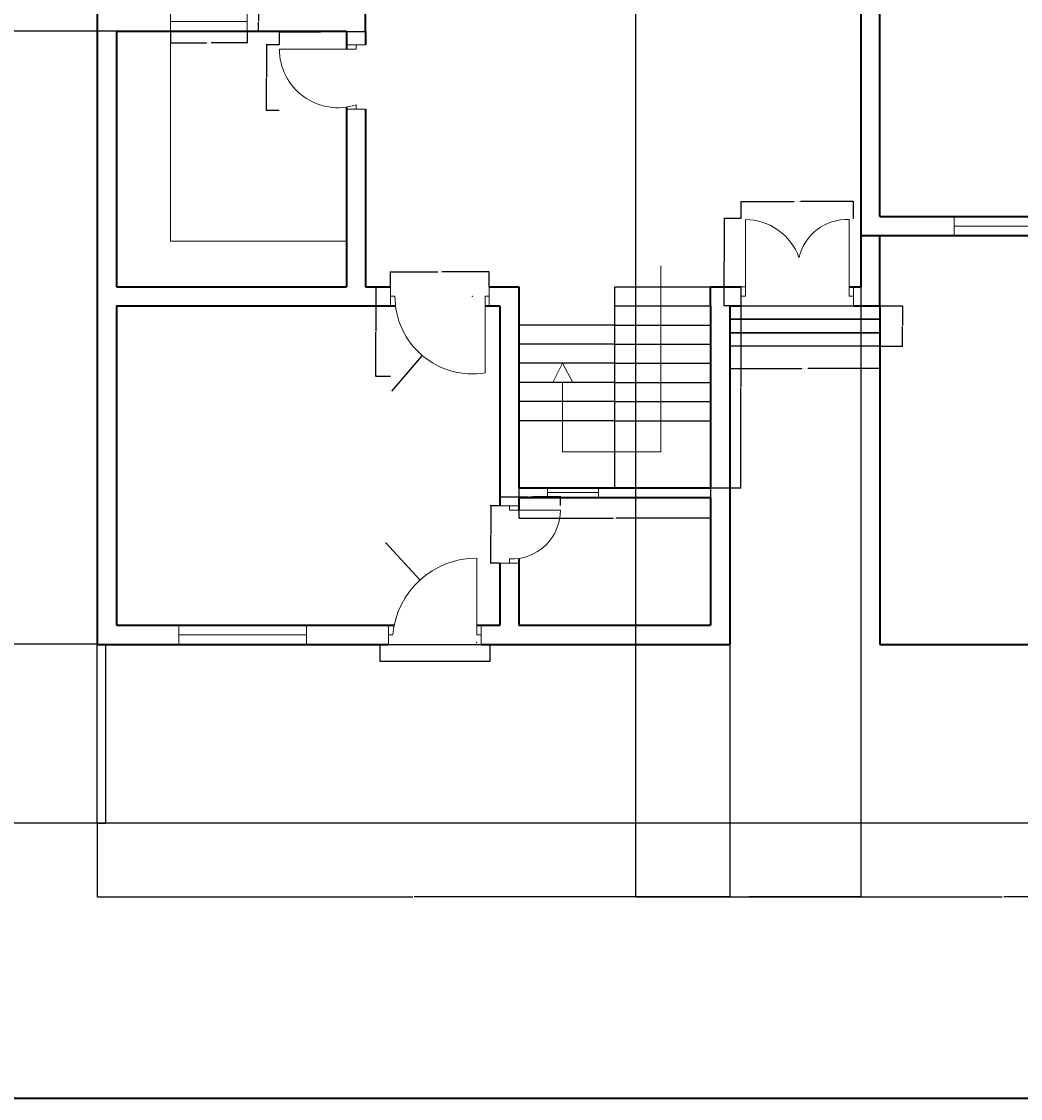
# Model space of a CAD drawing. Units: inches. Extents: x 2014 to 3678, y 870 to 2323.
# Tile 4 of 7: x 2813 to 3282, y 870 to 1376. Entities that reach past the tile are written whole.
import ezdxf

# ---------------------------------------------------------------- set-up
doc = ezdxf.new("R2010")
doc.units = ezdxf.units.IN
for name, color, linetype, lineweight in [('A-ANNO-DIMS', 2, 'Continuous', 18), ('A-ANNO-SYMB', 2, 'Continuous', 18), ('A-ANNO-TTLB', 7, 'Continuous', 35), ('A-DOOR', 3, 'Continuous', 18), ('A-FLOR-FIXT', 8, 'Continuous', 18), ('A-FLOR-STRS', 7, 'Continuous', 25), ('A-GLAZ', 4, 'Continuous', 18), ('A-SITE', 8, 'Continuous', 25), ('A-WALL', 7, 'Continuous', 35)]:
    doc.layers.add(name, color=color, linetype=linetype, lineweight=lineweight)
doc.styles.get("Standard").update_dxf_attribs({"font": 'arial.ttf'})
doc.dimstyles.get("Standard").update_dxf_attribs({"dimtxt": 0.18, "dimasz": 0.18, "dimexe": 0.18, "dimexo": 0.0625, "dimgap": 0.09, "dimtad": 0, "dimtih": 1, "dimtoh": 1, "dimdec": 4, "dimzin": 0, "dimdsep": 46, "dimtxsty": 'Standard', "dimcen": 0.09, "dimadec": 0, "dimazin": 0, "dimtfac": 1, "dimtdec": 4, "dimtofl": 0, "dimtmove": 0, "dimatfit": 3, "dimfxl": 1, "dimtolj": 1, "dimtzin": 0, "dimarcsym": 0})

# ---------------------------------------------------------------- blocks, each defined once
blk = doc.blocks.new('DOOR-DRAWING-36')
for p, q in [((0, 40.98), (0, 31.98)), ((46.34, 40.98), (46.34, 31.98)), ((0, 31.98), (0, 36.48)), ((0, 36.48), (2, 36.48)), ((46.34, 36.48), (44.34, 36.48)), ((44.34, 36.48), (44.34, 0.48)), ((46.34, 31.98), (46.34, 36.48))]:
    blk.add_line(p, q)
blk.add_arc((38.48, 36.48), 36.48, 180, 279.258)
blk = doc.blocks.new('DOOR-BATH-FRONT-24')
for p, q in [((0, 27), (9, 27)), ((9, 27), (4.5, 27)), ((4.5, 27), (4.5, 25)), ((4.5, 25), (28.5, 25)), ((4.5, 0), (4.5, 2)), ((0, 0), (9, 0)), ((9, 0), (4.5, 0))]:
    blk.add_line(p, q)
blk.add_arc((5.48, 25), 23.02, 267.569, 0)
blk = doc.blocks.new('DOOR-FRONT-36')
for p, q in [((41.48, 4.5), (41.48, 40.5)), ((0, 9), (0, 0)), ((43.48, 9), (43.48, 0)), ((0, 0), (0, 4.5)), ((0, 4.5), (2, 4.5)), ((43.48, 4.5), (41.48, 4.5)), ((43.48, 0), (43.48, 4.5))]:
    blk.add_line(p, q)
blk.add_arc((41.48, 0.85), 39.65, 90, 174.7231)
blk = doc.blocks.new('DOOR-KITCHEN-36')
for p, q in [((12, 28.21), (0, 28.21)), ((36, 28.21), (12, 28.21)), ((31.5, 30.21), (40.5, 30.21)), ((40.5, 30.21), (36, 30.21)), ((36, 30.21), (36, 28.21)), ((36, 0), (36, 2)), ((40.5, 0), (31.5, 0)), ((31.5, 0), (36, 0))]:
    blk.add_line(p, q)
blk.add_arc((27.54, 28.21), 27.54, 180, 287.8943)
blk = doc.blocks.new('WIN-60')
for p, q in [((0, 9), (0, 0)), ((60, 4.5), (60, 9)), ((60, 9), (60, 0)), ((0, 0), (0, 4.5)), ((0, 4.5), (60, 4.5))]:
    blk.add_line(p, q)
blk = doc.blocks.new('VENT-24')
for p, q in [((0, 24), (4.5, 24)), ((4.5, 24), (2.25, 24)), ((2.25, 24), (2.25, 0)), ((2.25, 0), (0, 0)), ((0, 0), (4.5, 0))]:
    blk.add_line(p, q)
blk = doc.blocks.new('WIN-36')
for p, q in [((0, 9), (0, 0)), ((36, 0), (36, 9)), ((0, 0), (0, 4.5)), ((0, 4.5), (36, 4.5)), ((36, 4.5), (36, 0))]:
    blk.add_line(p, q)
blk = doc.blocks.new('STAIR-HALF-TURN')
for p, q in [((45, 0), (45, 94.5)), ((45, 94.5), (90, 94.5)), ((45, 85.5), (90, 85.5)), ((45, 76.5), (0, 76.5)), ((45, 76.5), (90, 76.5)), ((45, 67.5), (0, 67.5)), ((45, 67.5), (90, 67.5)), ((45, 58.5), (0, 58.5)), ((45, 58.5), (90, 58.5)), ((45, 49.5), (0, 49.5)), ((45, 49.5), (90, 49.5)), ((45, 40.5), (0, 40.5)), ((45, 40.5), (90, 40.5)), ((45, 31.5), (0, 31.5)), ((45, 31.5), (90, 31.5)), ((90, 0), (0, 0))]:
    blk.add_line(p, q)
blk = doc.blocks.new('STAIR-DIRECTION')
for p, q in [((50.73, 87.32), (50.73, 0)), ((4.61, 41.51), (0, 32.51)), ((9.52, 32.51), (4.61, 41.51)), ((0, 32.51), (9.52, 32.51)), ((4.61, 0), (4.61, 32.51)), ((50.73, 0), (4.61, 0))]:
    blk.add_line(p, q)
blk = doc.blocks.new('STEPS-LOBBY')
for points in [[(0, 18.9), (70.5, 18.9), (70.5, 12.6), (0, 12.6)], [(0, 12.6), (70.5, 12.6), (70.5, 6.3), (0, 6.3)], [(0, 6.3), (70.5, 6.3), (70.5, 0), (0, 0)]]:
    blk.add_lwpolyline(points, close=True)
blk = doc.blocks.new('COUNTER-KITCHEN-L')
for p, q in [((0, 98.61), (0, 0)), ((0, 0), (82.65, 0))]:
    blk.add_line(p, q)
blk = doc.blocks.new('DOOR-LOBBY-PAIR')
for p, q in [((2, 4.5), (2, 40.5)), ((50.71, 4.5), (50.71, 40.5)), ((0, 9), (0, 0)), ((0, 9), (2, 9)), ((52.71, 9), (52.71, 0)), ((0, 4.5), (2, 4.5)), ((52.71, 4.5), (50.71, 4.5)), ((52.71, 0), (52.71, 4.5))]:
    blk.add_line(p, q)
for centre, radius, start, end in [((2, 13.8), 26.7, 19.351, 90), ((49.6, 17.54), 22.98, 87.2318, 167.173)]:
    blk.add_arc(centre, radius, start, end)
blk = doc.blocks.new('*D46')
at = {"layer": 'A-ANNO-DIMS', "color": 0, "lineweight": -2, "transparency": 16777216}
for p, q in [((2986.41, 1251.23), (2986.41, 1258.3)), ((2986.59, 1258.12), (3008.65, 1258.12)), ((3032.58, 1258.12), (3010.52, 1258.12)), ((3032.76, 1251.23), (3032.76, 1258.3))]:
    blk.add_line(p, q, dxfattribs=at)
at = {"layer": 'A-ANNO-DIMS', "color": 0, "transparency": 16777216}
for points in [[(2986.59, 1258.15), (2986.59, 1258.09), (2986.41, 1258.12)], [(3032.58, 1258.15), (3032.58, 1258.09), (3032.76, 1258.12)]]:
    blk.add_solid(points, dxfattribs=at)
at = {"layer": 'Defpoints', "color": 0, "transparency": 16777216}
for p in [(3032.76, 1258.12), (2986.41, 1251.17), (3032.76, 1251.17)]:
    blk.add_point(p, dxfattribs=at)
at = {"layer": 'A-ANNO-DIMS', "color": 0, "transparency": 16777216, "insert": (3009.59, 1258.12), "char_height": 0.18, "attachment_point": 5}
blk.add_mtext('\\A1;DOOR 46 TYP.', dxfattribs=at)
blk = doc.blocks.new('*D47')
at = {"layer": 'A-ANNO-DIMS', "color": 0, "lineweight": -2, "transparency": 16777216}
for p, q in [((2986.35, 1251.17), (2979.28, 1251.17)), ((2979.46, 1250.99), (2979.46, 1230.24)), ((2979.46, 1209.12), (2979.46, 1229.87)), ((2986.35, 1208.94), (2979.28, 1208.94))]:
    blk.add_line(p, q, dxfattribs=at)
at = {"layer": 'A-ANNO-DIMS', "color": 0, "transparency": 16777216}
for points in [[(2979.43, 1250.99), (2979.49, 1250.99), (2979.46, 1251.17)], [(2979.43, 1209.12), (2979.49, 1209.12), (2979.46, 1208.94)]]:
    blk.add_solid(points, dxfattribs=at)
at = {"layer": 'Defpoints', "color": 0, "transparency": 16777216}
for p in [(2979.46, 1251.17), (2986.41, 1251.17), (2986.41, 1208.94)]:
    blk.add_point(p, dxfattribs=at)
at = {"layer": 'A-ANNO-DIMS', "color": 0, "transparency": 16777216, "insert": (2979.46, 1230.05), "char_height": 0.18, "attachment_point": 5}
blk.add_mtext('\\A1;42 TYP.', dxfattribs=at)
blk = doc.blocks.new('*D48')
at = {"layer": 'A-ANNO-DIMS', "color": 0, "lineweight": -2, "transparency": 16777216}
for p, q in [((3037.67, 1148.32), (3037.67, 1152.71)), ((3037.85, 1152.53), (3050.62, 1152.53)), ((3065.99, 1152.53), (3053.23, 1152.53)), ((3066.17, 1148.32), (3066.17, 1152.71))]:
    blk.add_line(p, q, dxfattribs=at)
at = {"layer": 'A-ANNO-DIMS', "color": 0, "transparency": 16777216}
for points in [[(3037.85, 1152.56), (3037.85, 1152.5), (3037.67, 1152.53)], [(3065.99, 1152.56), (3065.99, 1152.5), (3066.17, 1152.53)]]:
    blk.add_solid(points, dxfattribs=at)
at = {"layer": 'Defpoints', "color": 0, "transparency": 16777216}
for p in [(3066.17, 1152.53), (3037.67, 1148.26), (3066.17, 1148.26)]:
    blk.add_point(p, dxfattribs=at)
at = {"layer": 'A-ANNO-DIMS', "color": 0, "transparency": 16777216, "insert": (3051.92, 1152.53), "char_height": 0.18, "attachment_point": 5}
blk.add_mtext('\\A1;BATH DOOR 29 TYP.', dxfattribs=at)
blk = doc.blocks.new('*D49')
at = {"layer": 'A-ANNO-DIMS', "color": 0, "lineweight": -2, "transparency": 16777216}
for p, q in [((3037.61, 1148.26), (3033.22, 1148.26)), ((3033.4, 1148.08), (3033.4, 1134.94)), ((3033.4, 1121.43), (3033.4, 1134.57)), ((3037.61, 1121.25), (3033.22, 1121.25))]:
    blk.add_line(p, q, dxfattribs=at)
at = {"layer": 'A-ANNO-DIMS', "color": 0, "transparency": 16777216}
for points in [[(3033.37, 1148.08), (3033.43, 1148.08), (3033.4, 1148.26)], [(3033.37, 1121.43), (3033.43, 1121.43), (3033.4, 1121.25)]]:
    blk.add_solid(points, dxfattribs=at)
at = {"layer": 'Defpoints', "color": 0, "transparency": 16777216}
for p in [(3033.4, 1148.26), (3037.67, 1148.26), (3037.67, 1121.25)]:
    blk.add_point(p, dxfattribs=at)
at = {"layer": 'A-ANNO-DIMS', "color": 0, "transparency": 16777216, "insert": (3033.4, 1134.76), "char_height": 0.18, "attachment_point": 5}
blk.add_mtext('\\A1;27 TYP.', dxfattribs=at)
blk = doc.blocks.new('*D52')
at = {"layer": 'A-ANNO-DIMS', "color": 0, "lineweight": -2, "transparency": 16777216}
for p, q in [((2934.17, 1364.83), (2934.17, 1371.02)), ((2974.67, 1364.83), (2974.67, 1371.02)), ((2934.35, 1370.84), (2953.49, 1370.84)), ((2974.49, 1370.84), (2955.36, 1370.84))]:
    blk.add_line(p, q, dxfattribs=at)
at = {"layer": 'A-ANNO-DIMS', "color": 0, "transparency": 16777216}
for points in [[(2934.35, 1370.87), (2934.35, 1370.81), (2934.17, 1370.84)], [(2974.49, 1370.87), (2974.49, 1370.81), (2974.67, 1370.84)]]:
    blk.add_solid(points, dxfattribs=at)
at = {"layer": 'Defpoints', "color": 0, "transparency": 16777216}
for p in [(2974.67, 1370.84), (2934.17, 1364.76), (2974.67, 1364.76)]:
    blk.add_point(p, dxfattribs=at)
at = {"layer": 'A-ANNO-DIMS', "color": 0, "transparency": 16777216, "insert": (2954.42, 1370.84), "char_height": 0.18, "attachment_point": 5}
blk.add_mtext('\\A1;DOOR 41 TYP.', dxfattribs=at)
blk = doc.blocks.new('*D53')
at = {"layer": 'A-ANNO-DIMS', "color": 0, "lineweight": -2, "transparency": 16777216}
for p, q in [((2934.11, 1364.76), (2927.92, 1364.76)), ((2928.1, 1364.58), (2928.1, 1349.49)), ((2928.1, 1334.03), (2928.1, 1349.13)), ((2934.11, 1333.85), (2927.92, 1333.85))]:
    blk.add_line(p, q, dxfattribs=at)
at = {"layer": 'A-ANNO-DIMS', "color": 0, "transparency": 16777216}
for points in [[(2928.07, 1364.58), (2928.13, 1364.58), (2928.1, 1364.76)], [(2928.07, 1334.03), (2928.13, 1334.03), (2928.1, 1333.85)]]:
    blk.add_solid(points, dxfattribs=at)
at = {"layer": 'Defpoints', "color": 0, "transparency": 16777216}
for p in [(2928.1, 1364.76), (2934.17, 1364.76), (2934.17, 1333.85)]:
    blk.add_point(p, dxfattribs=at)
at = {"layer": 'A-ANNO-DIMS', "color": 0, "transparency": 16777216, "insert": (2928.1, 1349.31), "char_height": 0.18, "attachment_point": 5}
blk.add_mtext('\\A1;31 TYP.', dxfattribs=at)
blk = doc.blocks.new('*D54')
at = {"layer": 'A-ANNO-DIMS', "color": 0, "lineweight": -2, "transparency": 16777216}
for p, q in [((2883.02, 1371.1), (2883.02, 1365.59)), ((2919.02, 1371.1), (2919.02, 1365.59)), ((2883.2, 1365.77), (2899.91, 1365.77)), ((2918.84, 1365.77), (2902.14, 1365.77))]:
    blk.add_line(p, q, dxfattribs=at)
at = {"layer": 'A-ANNO-DIMS', "color": 0, "transparency": 16777216}
for points in [[(2883.2, 1365.8), (2883.2, 1365.74), (2883.02, 1365.77)], [(2918.84, 1365.8), (2918.84, 1365.74), (2919.02, 1365.77)]]:
    blk.add_solid(points, dxfattribs=at)
at = {"layer": 'Defpoints', "color": 0, "transparency": 16777216}
for p in [(2883.02, 1371.17), (2919.02, 1371.17), (2919.02, 1365.77)]:
    blk.add_point(p, dxfattribs=at)
at = {"layer": 'A-ANNO-DIMS', "color": 0, "transparency": 16777216, "insert": (2901.02, 1365.77), "char_height": 0.18, "attachment_point": 5}
blk.add_mtext('\\A1;WINDOW 36 TYP.', dxfattribs=at)
blk = doc.blocks.new('*D55')
at = {"layer": 'A-ANNO-DIMS', "color": 0, "lineweight": -2, "transparency": 16777216}
for p, q in [((2919.09, 1380.17), (2924.6, 1380.17)), ((2924.42, 1379.99), (2924.42, 1375.85)), ((2919.09, 1371.17), (2924.6, 1371.17)), ((2924.42, 1371.35), (2924.42, 1375.48))]:
    blk.add_line(p, q, dxfattribs=at)
at = {"layer": 'A-ANNO-DIMS', "color": 0, "transparency": 16777216}
for points in [[(2924.39, 1379.99), (2924.45, 1379.99), (2924.42, 1380.17)], [(2924.39, 1371.35), (2924.45, 1371.35), (2924.42, 1371.17)]]:
    blk.add_solid(points, dxfattribs=at)
at = {"layer": 'Defpoints', "color": 0, "transparency": 16777216}
for p in [(2919.02, 1380.17), (2924.42, 1380.17), (2919.02, 1371.17)]:
    blk.add_point(p, dxfattribs=at)
at = {"layer": 'A-ANNO-DIMS', "color": 0, "transparency": 16777216, "insert": (2924.42, 1375.67), "char_height": 0.18, "attachment_point": 5}
blk.add_mtext('\\A1;9 TYP.', dxfattribs=at)
blk = doc.blocks.new('*D64')
at = {"layer": 'A-ANNO-DIMS', "color": 0, "lineweight": -2, "transparency": 16777216}
for p, q in [((3136.73, 1251.17), (3151.03, 1251.17)), ((3150.85, 1250.99), (3150.85, 1204.1)), ((3150.85, 1156.85), (3150.85, 1203.73)), ((3136.73, 1156.67), (3151.03, 1156.67))]:
    blk.add_line(p, q, dxfattribs=at)
at = {"layer": 'A-ANNO-DIMS', "color": 0, "transparency": 16777216}
for points in [[(3150.82, 1250.99), (3150.88, 1250.99), (3150.85, 1251.17)], [(3150.82, 1156.85), (3150.88, 1156.85), (3150.85, 1156.67)]]:
    blk.add_solid(points, dxfattribs=at)
at = {"layer": 'Defpoints', "color": 0, "transparency": 16777216}
for p in [(3136.67, 1251.17), (3150.85, 1251.17), (3136.67, 1156.67)]:
    blk.add_point(p, dxfattribs=at)
at = {"layer": 'A-ANNO-DIMS', "color": 0, "transparency": 16777216, "insert": (3150.85, 1203.92), "char_height": 0.18, "attachment_point": 5}
blk.add_mtext('\\A1;STAIR 95 TYP.', dxfattribs=at)
blk = doc.blocks.new('*D65')
at = {"layer": 'A-ANNO-DIMS', "color": 0, "lineweight": -2, "transparency": 16777216}
for p, q in [((3046.67, 1156.6), (3046.67, 1142.31)), ((3136.67, 1156.6), (3136.67, 1142.31)), ((3046.85, 1142.49), (3091.14, 1142.49)), ((3136.49, 1142.49), (3092.2, 1142.49))]:
    blk.add_line(p, q, dxfattribs=at)
at = {"layer": 'A-ANNO-DIMS', "color": 0, "transparency": 16777216}
for points in [[(3046.85, 1142.52), (3046.85, 1142.46), (3046.67, 1142.49)], [(3136.49, 1142.52), (3136.49, 1142.46), (3136.67, 1142.49)]]:
    blk.add_solid(points, dxfattribs=at)
at = {"layer": 'Defpoints', "color": 0, "transparency": 16777216}
for p in [(3046.67, 1156.67), (3136.67, 1156.67), (3136.67, 1142.49)]:
    blk.add_point(p, dxfattribs=at)
at = {"layer": 'A-ANNO-DIMS', "color": 0, "transparency": 16777216, "insert": (3091.67, 1142.49), "char_height": 0.18, "attachment_point": 5}
blk.add_mtext('\\A1;90 TYP.', dxfattribs=at)
blk = doc.blocks.new('*D66')
at = {"layer": 'A-ANNO-DIMS', "color": 0, "lineweight": -2, "transparency": 16777216}
for p, q in [((3145.67, 1223.2), (3145.67, 1212.51)), ((3216.17, 1223.2), (3216.17, 1212.51)), ((3145.85, 1212.69), (3179.5, 1212.69)), ((3215.99, 1212.69), (3182.35, 1212.69))]:
    blk.add_line(p, q, dxfattribs=at)
at = {"layer": 'A-ANNO-DIMS', "color": 0, "transparency": 16777216}
for points in [[(3145.85, 1212.72), (3145.85, 1212.66), (3145.67, 1212.69)], [(3215.99, 1212.72), (3215.99, 1212.66), (3216.17, 1212.69)]]:
    blk.add_solid(points, dxfattribs=at)
at = {"layer": 'Defpoints', "color": 0, "transparency": 16777216}
for p in [(3145.67, 1223.26), (3216.17, 1223.26), (3216.17, 1212.69)]:
    blk.add_point(p, dxfattribs=at)
at = {"layer": 'A-ANNO-DIMS', "color": 0, "transparency": 16777216, "insert": (3180.92, 1212.69), "char_height": 0.18, "attachment_point": 5}
blk.add_mtext('\\A1;LOBBY STEPS 71 TYP.', dxfattribs=at)
blk = doc.blocks.new('*D67')
at = {"layer": 'A-ANNO-DIMS', "color": 0, "lineweight": -2, "transparency": 16777216}
for p, q in [((3216.23, 1242.17), (3226.93, 1242.17)), ((3226.75, 1241.99), (3226.75, 1232.9)), ((3226.75, 1223.44), (3226.75, 1232.53)), ((3216.23, 1223.26), (3226.93, 1223.26))]:
    blk.add_line(p, q, dxfattribs=at)
at = {"layer": 'A-ANNO-DIMS', "color": 0, "transparency": 16777216}
for points in [[(3226.72, 1241.99), (3226.78, 1241.99), (3226.75, 1242.17)], [(3226.72, 1223.44), (3226.78, 1223.44), (3226.75, 1223.26)]]:
    blk.add_solid(points, dxfattribs=at)
at = {"layer": 'Defpoints', "color": 0, "transparency": 16777216}
for p in [(3216.17, 1242.17), (3226.75, 1242.17), (3216.17, 1223.26)]:
    blk.add_point(p, dxfattribs=at)
at = {"layer": 'A-ANNO-DIMS', "color": 0, "transparency": 16777216, "insert": (3226.75, 1232.71), "char_height": 0.18, "attachment_point": 5}
blk.add_mtext('\\A1;19 TYP.', dxfattribs=at)
blk = doc.blocks.new('*D70')
at = {"layer": 'A-ANNO-DIMS', "color": 0, "lineweight": -2, "transparency": 16777216}
for p, q in [((3150.99, 1283.27), (3150.99, 1291.29)), ((3151.17, 1291.11), (3175.87, 1291.11)), ((3203.52, 1291.11), (3178.82, 1291.11)), ((3203.7, 1283.27), (3203.7, 1291.29))]:
    blk.add_line(p, q, dxfattribs=at)
at = {"layer": 'A-ANNO-DIMS', "color": 0, "transparency": 16777216}
for points in [[(3151.17, 1291.14), (3151.17, 1291.08), (3150.99, 1291.11)], [(3203.52, 1291.14), (3203.52, 1291.08), (3203.7, 1291.11)]]:
    blk.add_solid(points, dxfattribs=at)
at = {"layer": 'Defpoints', "color": 0, "transparency": 16777216}
for p in [(3203.7, 1291.11), (3150.99, 1283.2), (3203.7, 1283.2)]:
    blk.add_point(p, dxfattribs=at)
at = {"layer": 'A-ANNO-DIMS', "color": 0, "transparency": 16777216, "insert": (3177.34, 1291.11), "char_height": 0.18, "attachment_point": 5}
blk.add_mtext('\\A1;LOBBY DOORS 53 TYP.', dxfattribs=at)
blk = doc.blocks.new('*D71')
at = {"layer": 'A-ANNO-DIMS', "color": 0, "lineweight": -2, "transparency": 16777216}
for p, q in [((3150.92, 1283.2), (3142.9, 1283.2)), ((3143.08, 1283.02), (3143.08, 1262.87)), ((3143.08, 1242.35), (3143.08, 1262.5)), ((3150.92, 1242.17), (3142.9, 1242.17))]:
    blk.add_line(p, q, dxfattribs=at)
at = {"layer": 'A-ANNO-DIMS', "color": 0, "transparency": 16777216}
for points in [[(3143.05, 1283.02), (3143.11, 1283.02), (3143.08, 1283.2)], [(3143.05, 1242.35), (3143.11, 1242.35), (3143.08, 1242.17)]]:
    blk.add_solid(points, dxfattribs=at)
at = {"layer": 'Defpoints', "color": 0, "transparency": 16777216}
for p in [(3143.08, 1283.2), (3150.99, 1283.2), (3150.99, 1242.17)]:
    blk.add_point(p, dxfattribs=at)
at = {"layer": 'A-ANNO-DIMS', "color": 0, "transparency": 16777216, "insert": (3143.08, 1262.68), "char_height": 0.18, "attachment_point": 5}
blk.add_mtext('\\A1;41 TYP.', dxfattribs=at)
blk = doc.blocks.new('*D93')
at = {"layer": 'A-ANNO-DIMS', "color": 0, "lineweight": -2, "transparency": 16777216}
for p, q in [((2848.61, 1083.17), (2778.34, 1083.17)), ((2778.52, 1082.99), (2778.52, 1041.35)), ((2778.52, 999.35), (2778.52, 1040.98)), ((2848.61, 999.17), (2778.34, 999.17))]:
    blk.add_line(p, q, dxfattribs=at)
at = {"layer": 'A-ANNO-DIMS', "color": 0, "transparency": 16777216}
for points in [[(2778.49, 1082.99), (2778.55, 1082.99), (2778.52, 1083.17)], [(2778.49, 999.35), (2778.55, 999.35), (2778.52, 999.17)]]:
    blk.add_solid(points, dxfattribs=at)
at = {"layer": 'Defpoints', "color": 0, "transparency": 16777216}
for p in [(2778.52, 1083.17), (2848.67, 1083.17), (2848.67, 999.17)]:
    blk.add_point(p, dxfattribs=at)
at = {"layer": 'A-ANNO-DIMS', "color": 0, "transparency": 16777216, "insert": (2778.52, 1041.17), "char_height": 0.18, "attachment_point": 5}
blk.add_mtext('\\A1;84', dxfattribs=at)
blk = doc.blocks.new('*D94')
at = {"layer": 'A-ANNO-DIMS', "color": 0, "lineweight": -2, "transparency": 16777216}
for p, q in [((2857.61, 1371.17), (2778.34, 1371.17)), ((2778.52, 1370.99), (2778.52, 1227.35)), ((2778.52, 1083.35), (2778.52, 1226.98)), ((2848.61, 1083.17), (2778.34, 1083.17))]:
    blk.add_line(p, q, dxfattribs=at)
at = {"layer": 'A-ANNO-DIMS', "color": 0, "transparency": 16777216}
for points in [[(2778.49, 1370.99), (2778.55, 1370.99), (2778.52, 1371.17)], [(2778.49, 1083.35), (2778.55, 1083.35), (2778.52, 1083.17)]]:
    blk.add_solid(points, dxfattribs=at)
at = {"layer": 'Defpoints', "color": 0, "transparency": 16777216}
for p in [(2778.52, 1371.17), (2857.67, 1371.17), (2848.67, 1083.17)]:
    blk.add_point(p, dxfattribs=at)
at = {"layer": 'A-ANNO-DIMS', "color": 0, "transparency": 16777216, "insert": (2778.52, 1227.17), "char_height": 0.18, "attachment_point": 5}
blk.add_mtext('\\A1;288', dxfattribs=at)
blk = doc.blocks.new('*D95')
at = {"layer": 'A-ANNO-DIMS', "color": 0, "lineweight": -2, "transparency": 16777216}
for p, q in [((2848.61, 1440.17), (2778.34, 1440.17)), ((2778.52, 1439.99), (2778.52, 1405.85)), ((2778.52, 1371.35), (2778.52, 1405.48)), ((2857.61, 1371.17), (2778.34, 1371.17))]:
    blk.add_line(p, q, dxfattribs=at)
at = {"layer": 'A-ANNO-DIMS', "color": 0, "transparency": 16777216}
for points in [[(2778.49, 1439.99), (2778.55, 1439.99), (2778.52, 1440.17)], [(2778.49, 1371.35), (2778.55, 1371.35), (2778.52, 1371.17)]]:
    blk.add_solid(points, dxfattribs=at)
at = {"layer": 'Defpoints', "color": 0, "transparency": 16777216}
for p in [(2778.52, 1440.17), (2848.67, 1440.17), (2857.67, 1371.17)]:
    blk.add_point(p, dxfattribs=at)
at = {"layer": 'A-ANNO-DIMS', "color": 0, "transparency": 16777216, "insert": (2778.52, 1405.67), "char_height": 0.18, "attachment_point": 5}
blk.add_mtext('\\A1;69', dxfattribs=at)
blk = doc.blocks.new('*D98')
at = {"layer": 'A-ANNO-DIMS', "color": 0, "lineweight": -2, "transparency": 16777216}
for p, q in [((2848.67, 999.1), (2848.67, 964.34)), ((3145.67, 999.1), (3145.67, 964.34)), ((2848.85, 964.52), (2996.88, 964.52)), ((3145.49, 964.52), (2997.46, 964.52))]:
    blk.add_line(p, q, dxfattribs=at)
at = {"layer": 'A-ANNO-DIMS', "color": 0, "transparency": 16777216}
for points in [[(2848.85, 964.55), (2848.85, 964.49), (2848.67, 964.52)], [(3145.49, 964.55), (3145.49, 964.49), (3145.67, 964.52)]]:
    blk.add_solid(points, dxfattribs=at)
at = {"layer": 'Defpoints', "color": 0, "transparency": 16777216}
for p in [(2848.67, 999.17), (3145.67, 999.17), (3145.67, 964.52)]:
    blk.add_point(p, dxfattribs=at)
at = {"layer": 'A-ANNO-DIMS', "color": 0, "transparency": 16777216, "insert": (2997.17, 964.52), "char_height": 0.18, "attachment_point": 5}
blk.add_mtext('\\A1;297', dxfattribs=at)
blk = doc.blocks.new('*D99')
at = {"layer": 'A-ANNO-DIMS', "color": 0, "lineweight": -2, "transparency": 16777216}
for p, q in [((3145.67, 999.1), (3145.67, 964.34)), ((3402.17, 999.1), (3402.17, 964.34)), ((3145.85, 964.52), (3273.53, 964.52)), ((3401.99, 964.52), (3274.32, 964.52))]:
    blk.add_line(p, q, dxfattribs=at)
at = {"layer": 'A-ANNO-DIMS', "color": 0, "transparency": 16777216}
for points in [[(3145.85, 964.55), (3145.85, 964.49), (3145.67, 964.52)], [(3401.99, 964.55), (3401.99, 964.49), (3402.17, 964.52)]]:
    blk.add_solid(points, dxfattribs=at)
at = {"layer": 'Defpoints', "color": 0, "transparency": 16777216}
for p in [(3145.67, 999.17), (3402.17, 999.17), (3402.17, 964.52)]:
    blk.add_point(p, dxfattribs=at)
at = {"layer": 'A-ANNO-DIMS', "color": 0, "transparency": 16777216, "insert": (3273.92, 964.52), "char_height": 0.18, "attachment_point": 5}
blk.add_mtext('\\A1;256.5', dxfattribs=at)
blk = doc.blocks.new('*D100')
at = {"layer": 'A-ANNO-DIMS', "color": 0, "lineweight": -2, "transparency": 16777216}
for p, q in [((3101.37, 1440.1), (3101.37, 964.34)), ((3207.17, 1427.25), (3207.17, 964.34)), ((3101.55, 964.52), (3153.88, 964.52)), ((3206.99, 964.52), (3154.65, 964.52))]:
    blk.add_line(p, q, dxfattribs=at)
at = {"layer": 'A-ANNO-DIMS', "color": 0, "transparency": 16777216}
for points in [[(3101.55, 964.55), (3101.55, 964.49), (3101.37, 964.52)], [(3206.99, 964.55), (3206.99, 964.49), (3207.17, 964.52)]]:
    blk.add_solid(points, dxfattribs=at)
at = {"layer": 'Defpoints', "color": 0, "transparency": 16777216}
for p in [(3101.37, 1440.17), (3207.17, 1427.31), (3207.17, 964.52)]:
    blk.add_point(p, dxfattribs=at)
at = {"layer": 'A-ANNO-DIMS', "color": 0, "transparency": 16777216, "insert": (3154.27, 964.52), "char_height": 0.18, "attachment_point": 5}
blk.add_mtext('\\A1;105.8', dxfattribs=at)
blk = doc.blocks.new('*D120')
at = {"layer": 'A-ANNO-DIMS', "color": 0, "lineweight": -2, "transparency": 16777216}
for p, q in [((2983.96, 1130.89), (2984.14, 1130.89)), ((2984.14, 1130.89), (3000.05, 1113.45)), ((3026.79, 1084.02), (3026.97, 1084.02)), ((3026.88, 1083.93), (3026.88, 1084.11))]:
    blk.add_line(p, q, dxfattribs=at)
at = {"layer": 'A-ANNO-DIMS', "color": 0, "transparency": 16777216}
blk.add_solid([(3000.07, 1113.47), (3000.03, 1113.43), (3000.17, 1113.31)], dxfattribs=at)
at = {"layer": 'Defpoints', "color": 0, "transparency": 16777216}
for p in [(3000.17, 1113.31), (3026.88, 1084.02)]:
    blk.add_point(p, dxfattribs=at)
at = {"layer": 'A-ANNO-DIMS', "color": 0, "transparency": 16777216, "insert": (2983.48, 1130.89), "char_height": 0.18, "attachment_point": 5}
blk.add_mtext('\\A1;R39.65', dxfattribs=at)
blk = doc.blocks.new('*D123')
at = {"layer": 'A-ANNO-DIMS', "color": 0, "lineweight": -2, "transparency": 16777216}
for p, q in [((3024.8, 1246.67), (3024.98, 1246.67)), ((3024.89, 1246.58), (3024.89, 1246.76)), ((2987.09, 1202.2), (3001.15, 1218.74)), ((2986.91, 1202.2), (2987.09, 1202.2))]:
    blk.add_line(p, q, dxfattribs=at)
at = {"layer": 'A-ANNO-DIMS', "color": 0, "transparency": 16777216}
blk.add_solid([(3001.12, 1218.76), (3001.17, 1218.72), (3001.26, 1218.88)], dxfattribs=at)
at = {"layer": 'Defpoints', "color": 0, "transparency": 16777216}
for p in [(3024.89, 1246.67), (3001.26, 1218.88)]:
    blk.add_point(p, dxfattribs=at)
at = {"layer": 'A-ANNO-DIMS', "color": 0, "transparency": 16777216, "insert": (2986.36, 1202.2), "char_height": 0.18, "attachment_point": 5}
blk.add_mtext('\\A1;R36.475', dxfattribs=at)

msp = doc.modelspace()

# ---------------------------------------------------------------- linework, layer by layer
at = {"layer": 'A-ANNO-TTLB'}
msp.add_lwpolyline([(2014.0556, 2323.3638), (3678.0069, 2323.3638), (3678.0069, 869.855), (2014.0556, 869.855)], close=True, dxfattribs=at)
at = {"layer": 'A-FLOR-STRS'}
msp.add_lwpolyline([(2981.4546, 1083.1655), (3033.0378, 1083.1655), (3033.0378, 1075.091), (2981.4546, 1075.091)], close=True, dxfattribs=at)
at = {"layer": 'A-SITE'}
for p, q in [((2848.6718, 999.1655), (2848.6718, 1083.1655)), ((2852.6718, 999.1655), (2852.6718, 1083.1655)), ((3145.6718, 1083.1655), (3145.6718, 999.1655)), ((3402.1718, 999.1655), (2848.6718, 999.1655)), ((2848.6718, 999.1655), (2850.6718, 999.1655)), ((2850.6718, 999.1655), (2852.6718, 999.1655))]:
    msp.add_line(p, q, dxfattribs=at)
at = {"layer": 'A-WALL'}
for p, q in [((2848.6718, 1683.1655), (2848.6718, 1083.1655)), ((2974.6718, 1371.1655), (2974.8253, 1440.1655)), ((3207.1718, 1391.2811), (3207.1718, 1275.1655)), ((3216.1718, 1284.1655), (3216.1718, 1393.0704)), ((2857.6718, 1371.1655), (2965.6718, 1371.1655)), ((2857.6718, 1371.1655), (2857.6718, 1251.1655)), ((2857.6718, 1371.1655), (2965.6718, 1371.1655)), ((2965.6718, 1371.1655), (2965.6718, 1362.764)), ((2974.6718, 1371.1655), (2974.6718, 1364.764)), ((2965.6718, 1335.512), (2965.6718, 1251.1655)), ((2974.6718, 1334.5577), (2974.6718, 1251.1655)), ((3216.1718, 1284.1655), (3393.1718, 1284.1655)), ((3207.1718, 1275.1655), (3216.1718, 1275.1655)), ((3207.1718, 1275.1655), (3207.1718, 1251.1655)), ((3216.1718, 1275.1655), (3393.1718, 1275.1655)), ((3216.1718, 1242.1655), (3216.1718, 1275.1655)), ((2857.6718, 1251.1655), (2965.6718, 1251.1655)), ((2974.6718, 1251.1655), (2986.414, 1251.1655)), ((3032.7572, 1251.1655), (3046.6718, 1251.1655)), ((3046.6718, 1251.1655), (3046.6718, 1242.1655)), ((3136.6718, 1242.1655), (3136.6718, 1251.1655)), ((3136.6718, 1251.1655), (3150.986, 1251.1655)), ((3201.6978, 1251.1655), (3207.1718, 1251.1655)), ((2857.6718, 1242.1655), (2857.6718, 1092.1655)), ((2857.6718, 1242.1655), (2965.6718, 1242.1655)), ((2965.6718, 1242.1655), (2974.6718, 1242.1655)), ((2974.6718, 1242.1655), (2988.6926, 1242.1655)), ((3030.7572, 1242.1655), (3037.6718, 1242.1655)), ((3037.6718, 1242.1655), (3037.6718, 1148.2566)), ((3046.6718, 1242.1655), (3046.6718, 1156.6655)), ((3136.6718, 1242.1655), (3136.6718, 1156.6655)), ((3145.6718, 1242.1655), (3145.6718, 1083.1655)), ((3145.6718, 1242.1655), (3150.986, 1242.1655)), ((3203.6978, 1242.1655), (3207.1718, 1242.1655)), ((3207.1718, 1242.1655), (3216.1718, 1242.1655)), ((3216.1718, 1242.1655), (3216.1718, 1083.1655)), ((3046.6718, 1156.6655), (3136.6718, 1156.6655)), ((3046.6718, 1152.1655), (3046.6718, 1146.2566)), ((3046.6718, 1152.1655), (3136.6718, 1152.1655)), ((3136.6718, 1152.1655), (3136.6718, 1092.1655)), ((3046.6718, 1123.5044), (3046.6718, 1092.1655)), ((3037.6718, 1121.2539), (3037.6718, 1092.1655)), ((2857.6718, 1092.1655), (2988.084, 1092.1655)), ((3026.8843, 1092.1655), (3037.6718, 1092.1655)), ((3046.6718, 1092.1655), (3136.6718, 1092.1655)), ((2848.6718, 1083.1655), (2985.4061, 1083.1655)), ((3028.8843, 1083.1655), (3046.6718, 1083.1655)), ((3046.6718, 1083.1655), (3145.6718, 1083.1655)), ((3216.1718, 1083.1655), (3402.1718, 1083.1655))]:
    msp.add_line(p, q, dxfattribs=at)

# ---------------------------------------------------------------- block references
at = {"layer": 'A-ANNO-SYMB'}
msp.add_blockref('STAIR-DIRECTION', (3062.5281, 1173.658), dxfattribs=at)
at = {"layer": 'A-DOOR'}
for name, p in [('DOOR-KITCHEN-36', (2934.1721, 1334.558)), ('DOOR-LOBBY-PAIR', (3150.9861, 1242.165)), ('DOOR-DRAWING-36', (2986.4141, 1210.19)), ('DOOR-BATH-FRONT-24', (3037.6721, 1121.254)), ('DOOR-FRONT-36', (2985.4061, 1083.165))]:
    msp.add_blockref(name, p, dxfattribs=at)
at = {"layer": 'A-FLOR-FIXT'}
msp.add_blockref('COUNTER-KITCHEN-L', (2883.0251, 1272.556), dxfattribs=at)
at = {"layer": 'A-FLOR-STRS'}
for name, p in [('STAIR-HALF-TURN', (3046.6721, 1156.665)), ('STEPS-LOBBY', (3145.6721, 1223.263))]:
    msp.add_blockref(name, p, dxfattribs=at)
at = {"layer": 'A-GLAZ'}
for name, p in [('WIN-36', (2883.0251, 1371.165)), ('WIN-60', (3251.1162, 1275.165)), ('WIN-60', (2886.9711, 1083.165))]:
    msp.add_blockref(name, p, dxfattribs=at)
at = {"layer": 'A-GLAZ', "extrusion": (0, 0, -1), "zscale": -1, "rotation": 90}
msp.add_blockref('VENT-24', (-3060.031, 1152.1658), dxfattribs=at)

# ---------------------------------------------------------------- dimensions: what is measured, and where the dimension line sits
at = {"layer": 'A-ANNO-DIMS'}
for base, p1, p2, picture, middle in [((2778.5231, 1440.1655), (2857.6718, 1371.1655), (2848.6718, 1440.1655), '*D95', (2778.5231, 1405.6655)), ((2778.5231, 1371.1655), (2848.6718, 1083.1655), (2857.6718, 1371.1655), '*D94', (2778.5231, 1227.1655)), ((2778.5231, 1083.1655), (2848.6718, 999.1655), (2848.6718, 1083.1655), '*D93', (2778.5231, 1041.1655))]:
    dim = msp.add_linear_dim(base=base, p1=p1, p2=p2, angle=90, dimstyle='Standard', override={"dimdec": 0, "dimlfac": 1, "dimrnd": 0, "dimzin": 0, "dimdsep": 46, "dimlunit": 2}, dxfattribs=at)
    dim.commit()
    dim.dimension.update_dxf_attribs({"geometry": picture, "text_midpoint": middle})
for base, p1, p2, override, picture, middle in [((3207.1718, 964.5155), (3101.3665, 1440.1655), (3207.1718, 1427.3075), {"dimdec": 1, "dimlfac": 1, "dimrnd": 0, "dimzin": 0, "dimdsep": 46, "dimlunit": 2}, '*D100', (3154.2691, 964.5155)), ((3145.6718, 964.5155), (2848.6718, 999.1655), (3145.6718, 999.1655), {"dimdec": 0, "dimlfac": 1, "dimrnd": 0, "dimzin": 0, "dimdsep": 46, "dimlunit": 2}, '*D98', (2997.1718, 964.5155)), ((3402.1718, 964.5155), (3145.6718, 999.1655), (3402.1718, 999.1655), {"dimdec": 1, "dimlfac": 1, "dimrnd": 0, "dimzin": 0, "dimdsep": 46, "dimlunit": 2}, '*D99', (3273.9218, 964.5155))]:
    dim = msp.add_linear_dim(base=base, p1=p1, p2=p2, dimstyle='Standard', override=override, dxfattribs=at)
    dim.commit()
    dim.dimension.update_dxf_attribs({"geometry": picture, "text_midpoint": middle})
for base, p1, p2, text, picture, middle in [((2924.4246, 1380.1655), (2919.0246, 1371.1655), (2919.0246, 1380.1655), '<> TYP.', '*D55', (2924.4246, 1375.6655)), ((2928.0968, 1364.764), (2934.1718, 1333.8519), (2934.1718, 1364.764), '<> TYP.', '*D53', (2928.0968, 1349.3079)), ((3143.0792, 1283.2037), (3150.986, 1242.1655), (3150.986, 1283.2037), '<> TYP.', '*D71', (3143.0792, 1262.6846)), ((2979.4625, 1251.1655), (2986.414, 1208.9442), (2986.414, 1251.1655), '<> TYP.', '*D47', (2979.4625, 1230.0548)), ((3150.8467955134, 1251.1654745472), (3136.6717955133, 1156.6654745472), (3136.6717955133, 1251.1654745472), 'STAIR <> TYP.', '*D64', (3150.8467955134, 1203.9154745472)), ((3226.7468, 1242.1655), (3216.1718, 1223.263), (3216.1718, 1242.1655), '<> TYP.', '*D67', (3226.7468, 1232.7142)), ((3033.3968, 1148.2566), (3037.6718, 1121.2539), (3037.6718, 1148.2566), '<> TYP.', '*D49', (3033.3968, 1134.7553))]:
    dim = msp.add_linear_dim(base=base, p1=p1, p2=p2, angle=90, text=text, dimstyle='Standard', override={"dimdec": 0, "dimlfac": 1, "dimrnd": 0, "dimzin": 0, "dimdsep": 46, "dimlunit": 2}, dxfattribs=at)
    dim.commit()
    dim.dimension.update_dxf_attribs({"geometry": picture, "text_midpoint": middle})
for base, p1, p2, text, picture, middle in [((2919.0246, 1365.7655), (2883.0246, 1371.1655), (2919.0246, 1371.1655), 'WINDOW <> TYP.', '*D54', (2901.0246, 1365.7655)), ((2974.6717955133, 1370.8389775863), (2934.1717955133, 1364.7639775863), (2974.6717955133, 1364.7639775863), 'DOOR <> TYP.', '*D52', (2954.4217955133, 1370.8389775863)), ((3203.6978, 1291.1105), (3150.986, 1283.2037), (3203.6978, 1283.2037), 'LOBBY DOORS <> TYP.', '*D70', (3177.3419, 1291.1105)), ((3032.7572, 1258.117), (2986.414, 1251.1655), (3032.7572, 1251.1655), 'DOOR <> TYP.', '*D46', (3009.5856, 1258.117)), ((3216.1717955133, 1212.6880048684), (3145.6717955133, 1223.2630048684), (3216.1717955133, 1223.2630048684), 'LOBBY STEPS <> TYP.', '*D66', (3180.9217955133, 1212.6880048684)), ((3136.6718, 1142.4905), (3046.6718, 1156.6655), (3136.6718, 1156.6655), '<> TYP.', '*D65', (3091.6718, 1142.4905)), ((3066.1717955133, 1152.5316266635), (3037.6717955133, 1148.2566266635), (3066.1717955133, 1148.2566266635), 'BATH DOOR <> TYP.', '*D48', (3051.9217955133, 1152.5316266635))]:
    dim = msp.add_linear_dim(base=base, p1=p1, p2=p2, text=text, dimstyle='Standard', override={"dimdec": 0, "dimlfac": 1, "dimrnd": 0, "dimzin": 0, "dimdsep": 46, "dimlunit": 2}, dxfattribs=at)
    dim.commit()
    dim.dimension.update_dxf_attribs({"geometry": picture, "text_midpoint": middle})
for center, mpoint, override, picture, middle in [((3024.8891, 1246.6655), (3001.2631, 1218.8761), {"dimdec": 3, "dimlfac": 1, "dimrnd": 0, "dimzin": 0, "dimdsep": 46, "dimlunit": 2}, '*D123', (2986.3571, 1202.2025)), ((3026.8843, 1084.0192), (3000.1701, 1113.3139), {"dimdec": 2, "dimlfac": 1, "dimrnd": 0, "dimzin": 0, "dimdsep": 46, "dimlunit": 2}, '*D120', (2983.4811, 1130.8907))]:
    dim = msp.add_radius_dim(center=center, mpoint=mpoint, dimstyle='Standard', override=override, dxfattribs=at)
    dim.commit()
    dim.dimension.update_dxf_attribs({"geometry": picture, "text_midpoint": middle, "dimtype": 164})

doc.saveas('drawing.dxf')
